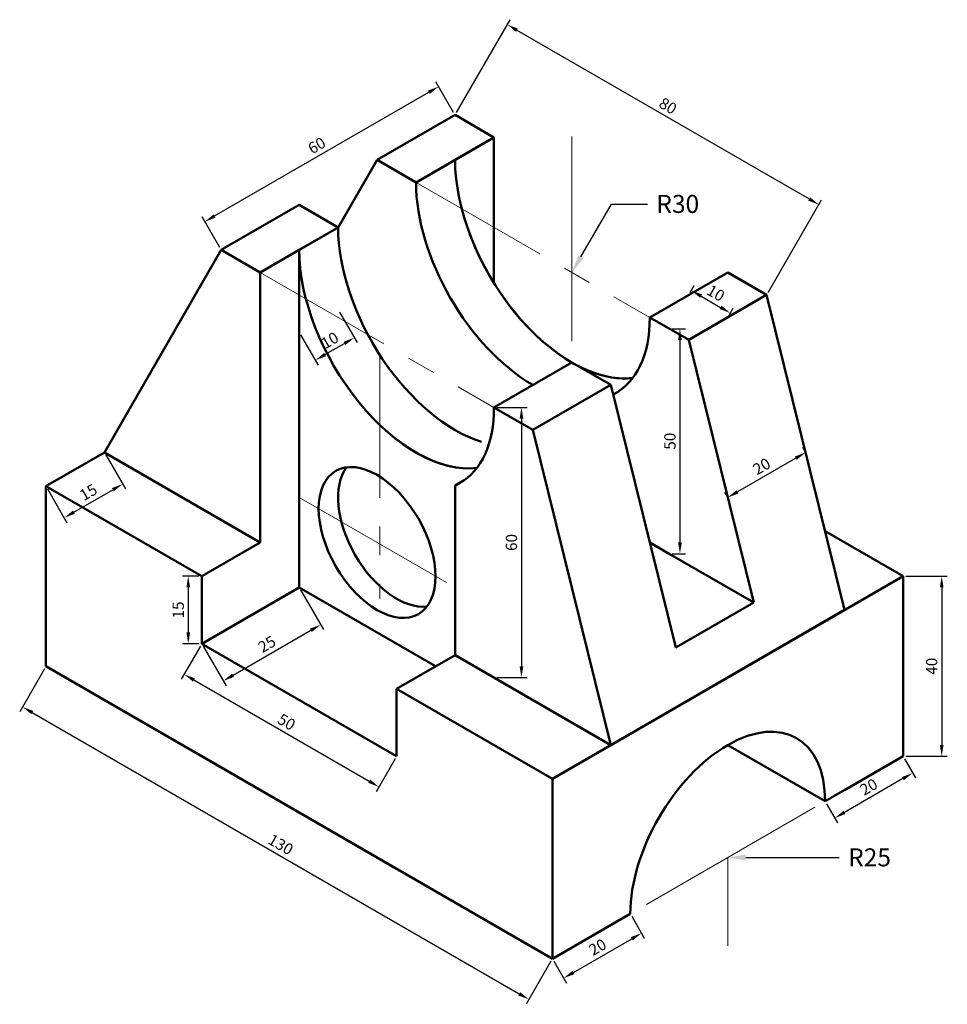
# Model space of a CAD drawing. Units: millimetres. Extents: x 2462 to 2668, y 2253 to 2472.
import ezdxf
from ezdxf import colors
from ezdxf.entities.mleader import LeaderData, LeaderLine
from ezdxf.math import Vec2, Vec3

# ---------------------------------------------------------------- set-up
doc = ezdxf.new("R2010")
doc.units = ezdxf.units.MM
doc.linetypes.add('CENTER', pattern=[50.8, 31.75, -6.35, 6.35, -6.35])
for name, color, linetype, lineweight in [('M-CNTR', 4, 'CENTER', 18), ('M-DIMS', 2, 'Continuous', 25), ('M-OUTL', 7, 'Continuous', 50)]:
    doc.layers.add(name, color=color, linetype=linetype, lineweight=lineweight)
doc.styles.get("Standard").update_dxf_attribs({"font": 'arial.ttf'})
doc.dimstyles.new('ISO-25', dxfattribs={"dimtxt": 2.5, "dimasz": 2.5, "dimexe": 1.25, "dimexo": 0.625, "dimtad": 1, "dimtxsty": 'Standard', "dimcen": 2.5, "dimadec": 0, "dimazin": 0, "dimtfac": 1, "dimtmove": 0, "dimatfit": 3, "dimfxl": 1, "dimarcsym": 0})

# ---------------------------------------------------------------- blocks, each defined once
blk = doc.blocks.new('*D1')
at = {"layer": 'Defpoints', "color": 0, "transparency": 16777216}
for p in [(2558.82, 2450.54), (2639.7, 2430.62), (2628.11, 2410.54)]:
    blk.add_point(p, dxfattribs=at)
at = {"layer": 'M-DIMS', "color": 0, "lineweight": -2, "transparency": 16777216}
for p, q in [((2559.14, 2451.08), (2571.05, 2471.71)), ((2572.59, 2469.37), (2637.54, 2431.87)), ((2628.42, 2411.08), (2640.33, 2431.71))]:
    blk.add_line(p, q, dxfattribs=at)
at = {"layer": 'M-DIMS', "color": 0, "transparency": 16777216}
for points in [[(2572.79, 2469.73), (2572.38, 2469.01), (2570.42, 2470.62)], [(2637.75, 2432.23), (2637.33, 2431.51), (2639.7, 2430.62)]]:
    blk.add_solid(points, dxfattribs=at)
at = {"layer": 'M-DIMS', "color": 0, "transparency": 16777216, "insert": (2606.01, 2452.27), "char_height": 2.5, "attachment_point": 5, "rotation": 330}
blk.add_mtext('80', dxfattribs=at)
blk = doc.blocks.new('*D2')
at = {"layer": 'Defpoints', "color": 0, "transparency": 16777216}
for p in [(2610.78, 2410.54), (2619.44, 2405.54), (2620.02, 2406.53)]:
    blk.add_point(p, dxfattribs=at)
at = {"layer": 'M-DIMS', "color": 0, "lineweight": -2, "transparency": 16777216}
for p, q in [((2611.1, 2411.08), (2611.99, 2412.62)), ((2613.53, 2410.28), (2617.86, 2407.78)), ((2619.76, 2406.08), (2620.65, 2407.62))]:
    blk.add_line(p, q, dxfattribs=at)
at = {"layer": 'M-DIMS', "color": 0, "transparency": 16777216}
for points in [[(2613.74, 2410.65), (2613.32, 2409.92), (2611.36, 2411.53)], [(2618.07, 2408.15), (2617.65, 2407.42), (2620.02, 2406.53)]]:
    blk.add_solid(points, dxfattribs=at)
at = {"layer": 'M-DIMS', "color": 0, "transparency": 16777216, "insert": (2616.64, 2410.68), "char_height": 2.5, "attachment_point": 5, "rotation": 330}
blk.add_mtext('10', dxfattribs=at)
blk = doc.blocks.new('*D3')
at = {"layer": 'Defpoints', "color": 0, "transparency": 16777216}
for p in [(2636.77, 2375.54), (2619.44, 2365.54), (2619.44, 2365.54)]:
    blk.add_point(p, dxfattribs=at)
at = {"layer": 'M-DIMS', "color": 0, "lineweight": -2, "transparency": 16777216}
for p, q in [((2636.45, 2376.08), (2636.14, 2376.62)), ((2634.6, 2374.29), (2621.61, 2366.79)), ((2619.13, 2366.08), (2618.82, 2366.62))]:
    blk.add_line(p, q, dxfattribs=at)
at = {"layer": 'M-DIMS', "color": 0, "transparency": 16777216}
for points in [[(2634.39, 2374.65), (2634.81, 2373.92), (2636.77, 2375.54)], [(2621.4, 2367.15), (2621.82, 2366.42), (2619.44, 2365.54)]]:
    blk.add_solid(points, dxfattribs=at)
at = {"layer": 'M-DIMS', "color": 0, "transparency": 16777216, "insert": (2627.15, 2372.18), "char_height": 2.5, "attachment_point": 5, "rotation": 30}
blk.add_mtext('20', dxfattribs=at)
blk = doc.blocks.new('*D4')
at = {"layer": 'Defpoints', "color": 0, "transparency": 16777216}
for p in [(2606.45, 2403.04), (2606.45, 2353.04), (2608.83, 2353.04)]:
    blk.add_point(p, dxfattribs=at)
at = {"layer": 'M-DIMS', "color": 0, "lineweight": -2, "transparency": 16777216}
for p, q in [((2607.08, 2403.04), (2610.08, 2403.04)), ((2608.83, 2400.54), (2608.83, 2355.54)), ((2607.08, 2353.04), (2610.08, 2353.04))]:
    blk.add_line(p, q, dxfattribs=at)
at = {"layer": 'M-DIMS', "color": 0, "transparency": 16777216}
for points in [[(2608.41, 2400.54), (2609.24, 2400.54), (2608.83, 2403.04)], [(2608.41, 2355.54), (2609.24, 2355.54), (2608.83, 2353.04)]]:
    blk.add_solid(points, dxfattribs=at)
at = {"layer": 'M-DIMS', "color": 0, "transparency": 16777216, "insert": (2606.92, 2378.04), "char_height": 2.5, "attachment_point": 5, "rotation": 90}
blk.add_mtext('50', dxfattribs=at)
blk = doc.blocks.new('*D5')
at = {"layer": 'Defpoints', "color": 0, "transparency": 16777216}
for p in [(2658.42, 2348.04), (2658.42, 2308.04), (2667.01, 2308.04)]:
    blk.add_point(p, dxfattribs=at)
at = {"layer": 'M-DIMS', "color": 0, "lineweight": -2, "transparency": 16777216}
for p, q in [((2659.04, 2348.04), (2668.26, 2348.04)), ((2667.01, 2345.54), (2667.01, 2310.54)), ((2659.04, 2308.04), (2668.26, 2308.04))]:
    blk.add_line(p, q, dxfattribs=at)
at = {"layer": 'M-DIMS', "color": 0, "transparency": 16777216}
for points in [[(2666.6, 2345.54), (2667.43, 2345.54), (2667.01, 2348.04)], [(2666.6, 2310.54), (2667.43, 2310.54), (2667.01, 2308.04)]]:
    blk.add_solid(points, dxfattribs=at)
at = {"layer": 'M-DIMS', "color": 0, "transparency": 16777216, "insert": (2665.11, 2328.04), "char_height": 2.5, "attachment_point": 5, "rotation": 90}
blk.add_mtext('40', dxfattribs=at)
blk = doc.blocks.new('*D6')
at = {"layer": 'Defpoints', "color": 0, "transparency": 16777216}
for p in [(2658.42, 2308.04), (2641.1, 2298.04), (2643.25, 2294.31)]:
    blk.add_point(p, dxfattribs=at)
at = {"layer": 'M-DIMS', "color": 0, "lineweight": -2, "transparency": 16777216}
for p, q in [((2658.73, 2307.49), (2661.19, 2303.23)), ((2658.4, 2303.06), (2645.41, 2295.56)), ((2641.41, 2297.49), (2643.87, 2293.23))]:
    blk.add_line(p, q, dxfattribs=at)
at = {"layer": 'M-DIMS', "color": 0, "transparency": 16777216}
for points in [[(2658.19, 2303.42), (2658.61, 2302.7), (2660.57, 2304.31)], [(2645.2, 2295.92), (2645.62, 2295.2), (2643.25, 2294.31)]]:
    blk.add_solid(points, dxfattribs=at)
at = {"layer": 'M-DIMS', "color": 0, "transparency": 16777216, "insert": (2650.96, 2300.96), "char_height": 2.5, "attachment_point": 5, "rotation": 30}
blk.add_mtext('20', dxfattribs=at)
blk = doc.blocks.new('*D7')
at = {"layer": 'Defpoints', "color": 0, "transparency": 16777216}
for p in [(2597.79, 2273.04), (2600.28, 2268.73), (2580.47, 2263.04)]:
    blk.add_point(p, dxfattribs=at)
at = {"layer": 'M-DIMS', "color": 0, "lineweight": -2, "transparency": 16777216}
for p, q in [((2598.11, 2272.49), (2600.91, 2267.64)), ((2585.13, 2259.98), (2598.12, 2267.48)), ((2580.79, 2262.49), (2583.59, 2257.64))]:
    blk.add_line(p, q, dxfattribs=at)
at = {"layer": 'M-DIMS', "color": 0, "transparency": 16777216}
for points in [[(2597.91, 2267.84), (2598.33, 2267.11), (2600.28, 2268.73)], [(2584.92, 2260.34), (2585.34, 2259.61), (2582.96, 2258.73)]]:
    blk.add_solid(points, dxfattribs=at)
at = {"layer": 'M-DIMS', "color": 0, "transparency": 16777216, "insert": (2590.67, 2265.37), "char_height": 2.5, "attachment_point": 5, "rotation": 30}
blk.add_mtext('20', dxfattribs=at)
blk = doc.blocks.new('*D8')
at = {"layer": 'Defpoints', "color": 0, "transparency": 16777216}
for p in [(2467.89, 2328.04), (2580.47, 2263.04), (2575.26, 2254)]:
    blk.add_point(p, dxfattribs=at)
at = {"layer": 'M-DIMS', "color": 0, "lineweight": -2, "transparency": 16777216}
for p, q in [((2467.58, 2327.49), (2462.05, 2317.92)), ((2464.84, 2317.75), (2573.09, 2255.25)), ((2580.16, 2262.49), (2574.63, 2252.92))]:
    blk.add_line(p, q, dxfattribs=at)
at = {"layer": 'M-DIMS', "color": 0, "transparency": 16777216}
for points in [[(2465.05, 2318.11), (2464.63, 2317.39), (2462.67, 2319)], [(2573.3, 2255.61), (2572.88, 2254.89), (2575.26, 2254)]]:
    blk.add_solid(points, dxfattribs=at)
at = {"layer": 'M-DIMS', "color": 0, "transparency": 16777216, "insert": (2519.92, 2288.15), "char_height": 2.5, "attachment_point": 5, "rotation": 330}
blk.add_mtext('130', dxfattribs=at)
blk = doc.blocks.new('*D9')
at = {"layer": 'Defpoints', "color": 0, "transparency": 16777216}
for p in [(2502.53, 2333.04), (2545.83, 2308.04), (2541.91, 2301.24)]:
    blk.add_point(p, dxfattribs=at)
at = {"layer": 'M-DIMS', "color": 0, "lineweight": -2, "transparency": 16777216}
for p, q in [((2502.22, 2332.49), (2497.98, 2325.15)), ((2500.77, 2324.99), (2539.74, 2302.49)), ((2545.52, 2307.49), (2541.28, 2300.15))]:
    blk.add_line(p, q, dxfattribs=at)
at = {"layer": 'M-DIMS', "color": 0, "transparency": 16777216}
for points in [[(2500.98, 2325.35), (2500.56, 2324.63), (2498.61, 2326.24)], [(2539.95, 2302.85), (2539.53, 2302.13), (2541.91, 2301.24)]]:
    blk.add_solid(points, dxfattribs=at)
at = {"layer": 'M-DIMS', "color": 0, "transparency": 16777216, "insert": (2521.21, 2315.38), "char_height": 2.5, "attachment_point": 5, "rotation": 330}
blk.add_mtext('50', dxfattribs=at)
blk = doc.blocks.new('*D10')
at = {"layer": 'Defpoints', "color": 0, "transparency": 16777216}
for p in [(2524.18, 2345.54), (2528.95, 2337.27), (2502.53, 2333.04)]:
    blk.add_point(p, dxfattribs=at)
at = {"layer": 'M-DIMS', "color": 0, "lineweight": -2, "transparency": 16777216}
for p, q in [((2524.49, 2344.99), (2529.58, 2336.19)), ((2509.47, 2326.02), (2526.79, 2336.02)), ((2502.84, 2332.49), (2507.93, 2323.69))]:
    blk.add_line(p, q, dxfattribs=at)
at = {"layer": 'M-DIMS', "color": 0, "transparency": 16777216}
for points in [[(2526.58, 2336.38), (2527, 2335.66), (2528.95, 2337.27)], [(2509.26, 2326.38), (2509.68, 2325.66), (2507.3, 2324.77)]]:
    blk.add_solid(points, dxfattribs=at)
at = {"layer": 'M-DIMS', "color": 0, "transparency": 16777216, "insert": (2517.18, 2332.67), "char_height": 2.5, "attachment_point": 5, "rotation": 30}
blk.add_mtext('25', dxfattribs=at)
blk = doc.blocks.new('*D11')
at = {"layer": 'Defpoints', "color": 0, "transparency": 16777216}
for p in [(2480.88, 2375.54), (2467.89, 2368.04), (2484.93, 2368.52)]:
    blk.add_point(p, dxfattribs=at)
at = {"layer": 'M-DIMS', "color": 0, "lineweight": -2, "transparency": 16777216}
for p, q in [((2481.19, 2374.99), (2485.55, 2367.44)), ((2468.2, 2367.49), (2472.56, 2359.94)), ((2474.1, 2362.27), (2482.76, 2367.27))]:
    blk.add_line(p, q, dxfattribs=at)
at = {"layer": 'M-DIMS', "color": 0, "transparency": 16777216}
for points in [[(2482.56, 2367.63), (2482.97, 2366.91), (2484.93, 2368.52)], [(2473.9, 2362.63), (2474.31, 2361.91), (2471.94, 2361.02)]]:
    blk.add_solid(points, dxfattribs=at)
at = {"layer": 'M-DIMS', "color": 0, "transparency": 16777216, "insert": (2477.48, 2366.42), "char_height": 2.5, "attachment_point": 5, "rotation": 30}
blk.add_mtext('15', dxfattribs=at)
blk = doc.blocks.new('*D12')
at = {"layer": 'Defpoints', "color": 0, "transparency": 16777216}
for p in [(2555.19, 2456.84), (2558.82, 2450.54), (2506.86, 2420.54)]:
    blk.add_point(p, dxfattribs=at)
at = {"layer": 'M-DIMS', "color": 0, "lineweight": -2, "transparency": 16777216}
for p, q in [((2558.51, 2451.08), (2554.56, 2457.92)), ((2505.39, 2428.09), (2553.02, 2455.59)), ((2506.55, 2421.08), (2502.6, 2427.92))]:
    blk.add_line(p, q, dxfattribs=at)
at = {"layer": 'M-DIMS', "color": 0, "transparency": 16777216}
for points in [[(2552.81, 2455.95), (2553.23, 2455.23), (2555.19, 2456.84)], [(2505.18, 2428.45), (2505.6, 2427.73), (2503.22, 2426.84)]]:
    blk.add_solid(points, dxfattribs=at)
at = {"layer": 'M-DIMS', "color": 0, "transparency": 16777216, "insert": (2528.25, 2443.48), "char_height": 2.5, "attachment_point": 5, "rotation": 30}
blk.add_mtext('60', dxfattribs=at)
blk = doc.blocks.new('*D13')
at = {"layer": 'Defpoints', "color": 0, "transparency": 16777216}
for p in [(2532.84, 2407.23), (2524.18, 2402.23), (2536.42, 2401.03)]:
    blk.add_point(p, dxfattribs=at)
at = {"layer": 'M-DIMS', "color": 0, "lineweight": -2, "transparency": 16777216}
for p, q in [((2533.15, 2406.69), (2537.04, 2399.95)), ((2524.49, 2401.69), (2528.38, 2394.95)), ((2529.92, 2397.28), (2534.25, 2399.78))]:
    blk.add_line(p, q, dxfattribs=at)
at = {"layer": 'M-DIMS', "color": 0, "transparency": 16777216}
for points in [[(2534.05, 2400.14), (2534.46, 2399.42), (2536.42, 2401.03)], [(2529.72, 2397.64), (2530.13, 2396.92), (2527.76, 2396.03)]]:
    blk.add_solid(points, dxfattribs=at)
at = {"layer": 'M-DIMS', "color": 0, "transparency": 16777216, "insert": (2531.14, 2400.18), "char_height": 2.5, "attachment_point": 5, "rotation": 30}
blk.add_mtext('10', dxfattribs=at)
blk = doc.blocks.new('*D14')
at = {"layer": 'Defpoints', "color": 0, "transparency": 16777216}
for p in [(2502.53, 2348.04), (2499.52, 2333.04), (2502.53, 2333.04)]:
    blk.add_point(p, dxfattribs=at)
at = {"layer": 'M-DIMS', "color": 0, "lineweight": -2, "transparency": 16777216}
for p, q in [((2501.91, 2348.04), (2498.27, 2348.04)), ((2499.52, 2345.54), (2499.52, 2335.54)), ((2501.91, 2333.04), (2498.27, 2333.04))]:
    blk.add_line(p, q, dxfattribs=at)
at = {"layer": 'M-DIMS', "color": 0, "transparency": 16777216}
for points in [[(2499.11, 2345.54), (2499.94, 2345.54), (2499.52, 2348.04)], [(2499.11, 2335.54), (2499.94, 2335.54), (2499.52, 2333.04)]]:
    blk.add_solid(points, dxfattribs=at)
at = {"layer": 'M-DIMS', "color": 0, "transparency": 16777216, "insert": (2497.62, 2340.54), "char_height": 2.5, "attachment_point": 5, "rotation": 90}
blk.add_mtext('15', dxfattribs=at)
blk = doc.blocks.new('*D15')
at = {"layer": 'Defpoints', "color": 0, "transparency": 16777216}
for p in [(2567.48, 2385.54), (2567.48, 2325.54), (2573.59, 2325.54)]:
    blk.add_point(p, dxfattribs=at)
at = {"layer": 'M-DIMS', "color": 0, "lineweight": -2, "transparency": 16777216}
for p, q in [((2568.11, 2385.54), (2574.84, 2385.54)), ((2573.59, 2383.04), (2573.59, 2328.04)), ((2568.11, 2325.54), (2574.84, 2325.54))]:
    blk.add_line(p, q, dxfattribs=at)
at = {"layer": 'M-DIMS', "color": 0, "transparency": 16777216}
for points in [[(2573.18, 2383.04), (2574.01, 2383.04), (2573.59, 2385.54)], [(2573.18, 2328.04), (2574.01, 2328.04), (2573.59, 2325.54)]]:
    blk.add_solid(points, dxfattribs=at)
at = {"layer": 'M-DIMS', "color": 0, "transparency": 16777216, "insert": (2571.69, 2355.54), "char_height": 2.5, "attachment_point": 5, "rotation": 90}
blk.add_mtext('60', dxfattribs=at)

msp = doc.modelspace()

# ---------------------------------------------------------------- linework, layer by layer
at = {"layer": 'M-CNTR'}
for p, q in [((2584.804, 2425.535), (2584.804, 2445.768)), ((2550.163, 2435.535), (2602.124, 2405.535)), ((2584.804, 2425.535), (2584.804, 2400.307)), ((2515.522, 2415.535), (2567.483, 2385.535)), ((2542.136, 2397.175), (2542.136, 2343.059)), ((2541.503, 2355.535), (2524.182, 2365.535)), ((2541.503, 2355.535), (2556.961, 2346.61)), ((2619.445, 2285.535), (2638.803, 2296.712)), ((2619.445, 2285.535), (2601.419, 2275.128)), ((2619.445, 2285.535), (2619.445, 2265.943))]:
    msp.add_line(p, q, dxfattribs=at)
at = {"layer": 'M-OUTL'}
for p, q in [((2558.823, 2450.535), (2541.503, 2440.535)), ((2541.503, 2440.535), (2558.823, 2450.535)), ((2567.483, 2445.535), (2558.823, 2450.535)), ((2550.163, 2435.535), (2567.483, 2445.535)), ((2567.483, 2445.535), (2550.163, 2435.535)), ((2567.483, 2445.535), (2550.163, 2435.535)), ((2567.483, 2445.535), (2558.823, 2440.535)), ((2567.483, 2413.174), (2567.483, 2445.535)), ((2541.503, 2440.535), (2532.842, 2425.535)), ((2541.503, 2440.535), (2550.163, 2435.535)), ((2506.862, 2420.535), (2524.182, 2430.535)), ((2506.862, 2420.535), (2524.182, 2430.535)), ((2524.182, 2430.535), (2532.842, 2425.535)), ((2532.842, 2425.535), (2515.522, 2415.535)), ((2532.842, 2425.535), (2524.182, 2420.535)), ((2506.862, 2420.535), (2480.881, 2375.535)), ((2515.522, 2415.535), (2506.862, 2420.535)), ((2515.522, 2415.535), (2524.182, 2420.535)), ((2524.182, 2345.535), (2524.182, 2420.535)), ((2515.522, 2355.535), (2515.522, 2415.535)), ((2515.522, 2355.535), (2515.522, 2415.535)), ((2619.445, 2415.535), (2602.124, 2405.535)), ((2628.105, 2410.535), (2619.445, 2415.535)), ((2610.785, 2400.535), (2628.105, 2410.535)), ((2645.426, 2340.535), (2628.105, 2410.535)), ((2602.124, 2405.535), (2610.785, 2400.535)), ((2524.182, 2345.535), (2524.182, 2402.228)), ((2524.182, 2386.375), (2524.182, 2402.228)), ((2625.218, 2342.202), (2610.785, 2400.535)), ((2584.804, 2395.535), (2567.483, 2385.535)), ((2593.464, 2390.535), (2584.804, 2395.535)), ((2576.144, 2380.535), (2593.464, 2390.535)), ((2576.144, 2380.535), (2593.464, 2390.535)), ((2607.898, 2332.202), (2593.464, 2390.535)), ((2567.483, 2385.535), (2576.144, 2380.535)), ((2576.144, 2380.535), (2593.464, 2310.535)), ((2467.891, 2368.035), (2480.881, 2375.535)), ((2480.881, 2375.535), (2515.522, 2355.535)), ((2502.532, 2348.035), (2467.891, 2368.035)), ((2467.891, 2328.035), (2467.891, 2368.035)), ((2558.823, 2368.174), (2560.868, 2369.355)), ((2558.823, 2330.535), (2558.823, 2368.174)), ((2524.182, 2345.535), (2524.182, 2365.535)), ((2524.182, 2345.535), (2524.182, 2365.535)), ((2658.416, 2348.035), (2641.096, 2358.035)), ((2502.532, 2348.035), (2515.522, 2355.535)), ((2606.455, 2353.035), (2602.124, 2355.535)), ((2606.455, 2353.035), (2625.218, 2342.202)), ((2502.532, 2333.035), (2502.532, 2348.035)), ((2580.474, 2303.035), (2658.416, 2348.035)), ((2593.464, 2310.535), (2658.416, 2348.035)), ((2658.416, 2308.035), (2658.416, 2348.035)), ((2502.532, 2333.035), (2524.182, 2345.535)), ((2502.532, 2333.035), (2524.182, 2345.535)), ((2524.182, 2345.535), (2554.493, 2328.035)), ((2625.218, 2342.202), (2607.898, 2332.202)), ((2593.464, 2310.535), (2645.426, 2340.535)), ((2593.464, 2310.535), (2645.426, 2340.535)), ((2645.426, 2340.535), (2628.105, 2330.535)), ((2545.833, 2308.035), (2502.532, 2333.035)), ((2545.833, 2323.035), (2558.823, 2330.535)), ((2558.823, 2330.535), (2593.464, 2310.535)), ((2467.891, 2328.035), (2580.474, 2263.035)), ((2545.833, 2308.035), (2545.833, 2323.035)), ((2580.474, 2303.035), (2545.833, 2323.035)), ((2545.833, 2323.035), (2545.833, 2308.035)), ((2593.464, 2310.535), (2610.785, 2320.535)), ((2641.096, 2298.035), (2619.445, 2310.535)), ((2545.833, 2283.035), (2502.532, 2308.035)), ((2641.096, 2298.035), (2658.416, 2308.035)), ((2641.096, 2298.035), (2658.416, 2308.035)), ((2658.416, 2308.035), (2641.096, 2298.035)), ((2645.426, 2300.535), (2658.416, 2308.035)), ((2580.474, 2263.035), (2580.474, 2303.035)), ((2524.182, 2295.535), (2545.833, 2283.035)), ((2580.474, 2263.035), (2597.794, 2273.035)), ((2580.474, 2263.035), (2597.794, 2273.035))]:
    msp.add_line(p, q, dxfattribs=at)
msp.add_arc((2569.492, 2400.601), 45.339, 177.94426, 182.05574, dxfattribs=at)
for centre, major_axis, start_param, end_param in [((2584.804, 2425.535), (18.371, -31.82), 3.9269908, 6.0452442), ((2576.144, 2420.535), (18.371, -31.82), 3.9269908, 5.4977871), ((2558.823, 2410.535), (18.371, -31.82), 3.9269908, 5.7263674), ((2584.804, 2425.535), (18.371, -31.82), 4.432994, 6.0452442), ((2550.163, 2405.535), (18.371, -31.82), 3.9269908, 6.0452442), ((2576.144, 2420.535), (18.371, -31.82), 6.2547876, 7.0685835), ((2541.503, 2400.535), (18.371, -31.82), 0, 0.7853982), ((2550.163, 2405.535), (18.371, -31.82), 5.2404833, 5.8376241), ((2545.833, 2358.035), (9.186, -15.91), 3.3795338, 6.0452442), ((2541.503, 2400.535), (18.371, -31.82), 6.2275148, 6.2831853), ((2619.445, 2285.535), (-15.309, -26.517), 2.3561945, 5.4977871)]:
    msp.add_ellipse(centre, major_axis=major_axis, ratio=0.5773503, start_param=start_param, end_param=end_param, dxfattribs=at)
msp.add_ellipse((2541.503, 2355.535), major_axis=(9.186, -15.91), ratio=0.5773503, dxfattribs=at)

# ---------------------------------------------------------------- dimensions: what is measured, and where the dimension line sits
at = {"layer": 'M-DIMS'}
for p1, p2, distance, picture, middle in [((2558.823, 2450.535), (2628.105, 2410.535), 23.196, '*D1', (2606.013, 2452.27)), ((2506.862, 2420.535), (2558.823, 2450.535), 7.276, '*D12', (2528.254, 2443.483)), ((2610.785, 2410.535), (2619.445, 2405.535), 1.154, '*D2', (2616.643, 2410.682)), ((2524.182, 2402.228), (2532.842, 2407.228), -7.154, '*D13', (2531.139, 2400.179)), ((2606.455, 2403.035), (2606.455, 2353.035), 2.37, '*D4', (2606.924, 2378.035)), ((2636.765, 2375.535), (2619.445, 2365.535), 0, '*D3', (2627.155, 2372.182)), ((2467.891, 2368.035), (2480.881, 2375.535), -8.096, '*D11', (2477.483, 2366.42)), ((2502.532, 2333.035), (2524.182, 2345.535), -9.545, '*D10', (2517.179, 2332.666)), ((2502.532, 2333.035), (2545.833, 2308.035), -7.85, '*D9', (2521.208, 2315.383)), ((2467.891, 2328.035), (2580.474, 2263.035), -10.434, '*D8', (2519.916, 2288.146)), ((2658.416, 2308.035), (2641.096, 2298.035), 4.301, '*D6', (2650.956, 2300.957)), ((2580.474, 2263.035), (2597.794, 2273.035), -4.976, '*D7', (2590.672, 2265.372))]:
    dim = msp.add_aligned_dim(p1=p1, p2=p2, distance=distance, dimstyle='ISO-25', override={"dimclrd": 0, "dimclre": 0, "dimclrt": 0}, dxfattribs=at)
    dim.commit()
    dim.dimension.update_dxf_attribs({"geometry": picture, "text_midpoint": middle})
for base, p1, p2, picture, middle in [((2573.593, 2325.535), (2567.483, 2385.535), (2567.483, 2325.535), '*D15', (2571.692, 2355.535)), ((2499.524, 2333.035), (2502.532, 2348.035), (2502.532, 2333.035), '*D14', (2497.622, 2340.535)), ((2667.015, 2308.035), (2658.416, 2348.035), (2658.416, 2308.035), '*D5', (2665.113, 2328.035))]:
    dim = msp.add_linear_dim(base=base, p1=p1, p2=p2, angle=90, dimstyle='ISO-25', override={"dimclrd": 0, "dimclre": 0, "dimclrt": 0}, dxfattribs=at)
    dim.commit()
    dim.dimension.update_dxf_attribs({"geometry": picture, "text_midpoint": middle})

# ---------------------------------------------------------------- leaders
ml = msp.add_multileader_mtext('Standard', dxfattribs=at)
ml.set_content('R30', color=256)
ml.set_leader_properties()
ml.build(insert=Vec2(0, 0))
ctx = ml.context
ctx.base_point, ctx.plane_origin = Vec3(2601.578, 2430.732), Vec3(2584.804, 2415.535)
notes = []
notes.append((ctx, [(0, (1, 1, 0), (2593.578, 2430.732), (1, 0), 8, [(0, [(2584.804, 2415.535)], 0, [])])]))
ctx.mtext.insert, ctx.mtext.flow_direction = Vec3(2603.578, 2432.768), 5
ml = msp.add_multileader_mtext('Standard', dxfattribs=at)
ml.set_content('R25', color=256)
ml.set_leader_properties()
ml.build(insert=Vec2(0, 0))
ctx = ml.context
ctx.base_point, ctx.plane_origin = Vec3(2644.21, 2285.535), Vec3(2619.445, 2285.535)
notes.append((ctx, [(0, (1, 1, 0), (2636.21, 2285.535), (1, 0), 8, [(0, [(2619.445, 2285.535)], 0, [])])]))
ctx.mtext.insert, ctx.mtext.flow_direction = Vec3(2646.21, 2287.569), 5
for ctx, leaders in notes:
    for number, flags, end, landing, length, lines in leaders:
        leader = LeaderData()
        leader.index, (leader.has_last_leader_line, leader.has_dogleg_vector, leader.attachment_direction) = number, flags
        leader.last_leader_point, leader.dogleg_vector, leader.dogleg_length = Vec3(end), Vec3(landing), length
        for number, points, colour, breaks in lines:
            line = LeaderLine()
            line.index, line.vertices, line.color, line.breaks = number, Vec3.list(points), colors.encode_raw_color(colour), breaks
            leader.lines.append(line)
        ctx.leaders.append(leader)

doc.saveas('drawing.dxf')
